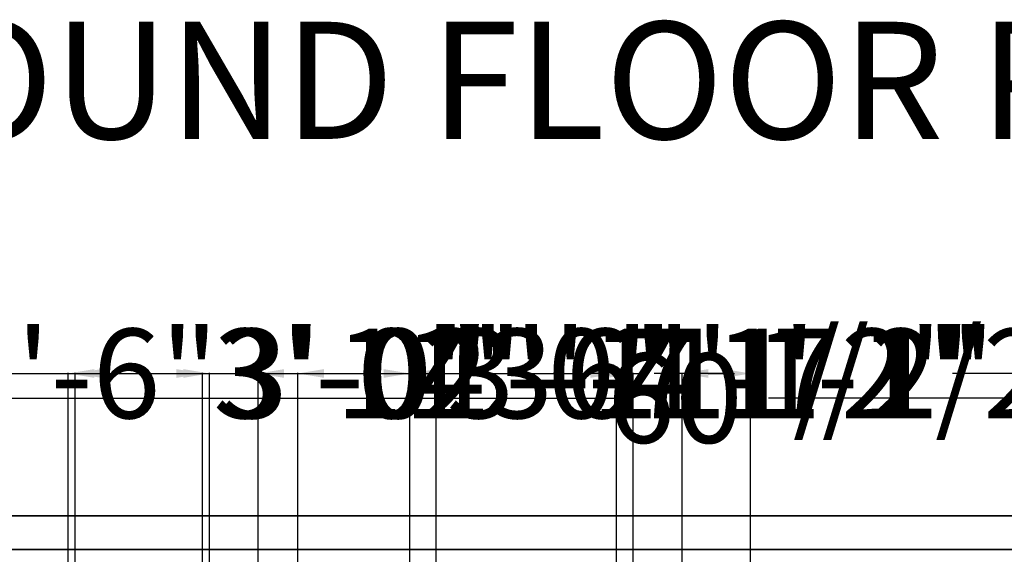
# Model space of a CAD drawing. Units: inches. Extents: x -166 to 1001, y 0 to 688.
# Tile 7 of 11: x 97 to 361, y 544 to 688. Entities that reach past the tile are written whole.
import ezdxf

# ---------------------------------------------------------------- set-up
doc = ezdxf.new("R2010")
doc.units = ezdxf.units.IN
doc.header["$MEASUREMENT"] = 0
for name, color, linetype, lineweight in [('A-ANNO-DIMS', 1, 'Continuous', 18), ('A-ANNO-TEXT', 2, 'Continuous', 25), ('C-SITE-WALL', 250, 'Continuous', 35)]:
    doc.layers.add(name, color=color, linetype=linetype, lineweight=lineweight)
doc.styles.get("Standard").update_dxf_attribs({"font": 'arial.ttf'})
doc.dimstyles.get("Standard").update_dxf_attribs({"dimtxt": 24, "dimasz": 7, "dimexe": 0.18, "dimexo": 0.0625, "dimgap": 0.09, "dimtad": 0, "dimtih": 1, "dimtoh": 1, "dimdec": 0, "dimzin": 0, "dimdsep": 46, "dimlunit": 3, "dimtxsty": 'Standard', "dimcen": 0.09, "dimadec": 0, "dimazin": 0, "dimtfac": 1, "dimtdec": 0, "dimtofl": 0, "dimtmove": 0, "dimatfit": 3, "dimfxl": 1, "dimtolj": 1, "dimtzin": 0, "dimarcsym": 0})

# ---------------------------------------------------------------- blocks, each defined once
blk = doc.blocks.new('*D10')
at = {"layer": 'A-ANNO-DIMS', "color": 0, "lineweight": -2, "transparency": 16777216}
for p, q in [((-82.62, 554.8), (-82.62, 586.48)), ((-75.62, 586.3), (256.61, 586.3)), ((629.88, 586.3), (297.65, 586.3)), ((636.88, 554.8), (636.88, 586.48))]:
    blk.add_line(p, q, dxfattribs=at)
at = {"layer": 'A-ANNO-DIMS', "color": 0, "transparency": 16777216}
for points in [[(-75.62, 587.47), (-75.62, 585.14), (-82.62, 586.3)], [(629.88, 587.47), (629.88, 585.14), (636.88, 586.3)]]:
    blk.add_solid(points, dxfattribs=at)
at = {"layer": 'Defpoints', "color": 0, "transparency": 16777216}
for p in [(636.88, 586.3), (-82.62, 554.74), (636.88, 554.74)]:
    blk.add_point(p, dxfattribs=at)
at = {"layer": 'A-ANNO-DIMS', "color": 0, "transparency": 16777216, "insert": (277.13, 586.3), "char_height": 24, "attachment_point": 5}
blk.add_mtext("\\A1;60'", dxfattribs=at)
blk = doc.blocks.new('*D35')
at = {"layer": 'A-ANNO-DIMS', "color": 0, "lineweight": -2, "transparency": 16777216}
for p, q in [((15.38, 483.8), (15.38, 593.07)), ((22.38, 592.89), (207.38, 592.89)), ((531.88, 592.89), (346.89, 592.89)), ((538.88, 483.8), (538.88, 593.07))]:
    blk.add_line(p, q, dxfattribs=at)
at = {"layer": 'A-ANNO-DIMS', "color": 0, "transparency": 16777216}
for points in [[(22.38, 594.06), (22.38, 591.72), (15.38, 592.89)], [(531.88, 594.06), (531.88, 591.72), (538.88, 592.89)]]:
    blk.add_solid(points, dxfattribs=at)
at = {"layer": 'Defpoints', "color": 0, "transparency": 16777216}
for p in [(538.88, 592.89), (15.38, 483.74), (538.88, 483.74)]:
    blk.add_point(p, dxfattribs=at)
at = {"layer": 'A-ANNO-DIMS', "color": 0, "transparency": 16777216, "insert": (277.13, 592.89), "char_height": 24, "attachment_point": 5}
blk.add_mtext('\\A1;43\'-7 1/2"', dxfattribs=at)
blk = doc.blocks.new('*D43')
at = {"layer": 'A-ANNO-DIMS', "color": 0, "lineweight": -2, "transparency": 16777216}
for p, q in [((160.88, 257.49), (160.88, 593.07)), ((167.88, 592.89), (201.62, 592.89)), ((208.62, 257.49), (208.62, 593.07)), ((208.62, 592.89), (215.62, 592.89))]:
    blk.add_line(p, q, dxfattribs=at)
at = {"layer": 'A-ANNO-DIMS', "color": 0, "transparency": 16777216}
for points in [[(167.88, 594.06), (167.88, 591.72), (160.88, 592.89)], [(201.62, 594.06), (201.62, 591.72), (208.62, 592.89)]]:
    blk.add_solid(points, dxfattribs=at)
at = {"layer": 'Defpoints', "color": 0, "transparency": 16777216}
for p in [(208.62, 592.89), (160.88, 257.42), (208.62, 257.42)]:
    blk.add_point(p, dxfattribs=at)
at = {"layer": 'A-ANNO-DIMS', "color": 0, "transparency": 16777216, "insert": (284.89, 592.89), "char_height": 24, "attachment_point": 5}
blk.add_mtext('\\A1;3\'-11 1/2"', dxfattribs=at)
blk = doc.blocks.new('*D59')
at = {"layer": 'A-ANNO-DIMS', "color": 0, "lineweight": -2, "transparency": 16777216}
for p, q in [((110.03, 342.8), (110.03, 593.07)), ((117.03, 592.89), (139.03, 592.89)), ((146.03, 342.8), (146.03, 593.07)), ((146.03, 592.89), (153.03, 592.89))]:
    blk.add_line(p, q, dxfattribs=at)
at = {"layer": 'A-ANNO-DIMS', "color": 0, "transparency": 16777216}
for points in [[(117.03, 594.06), (117.03, 591.72), (110.03, 592.89)], [(139.03, 594.06), (139.03, 591.72), (146.03, 592.89)]]:
    blk.add_solid(points, dxfattribs=at)
at = {"layer": 'Defpoints', "color": 0, "transparency": 16777216}
for p in [(146.03, 592.89), (110.03, 342.74), (146.03, 342.74)]:
    blk.add_point(p, dxfattribs=at)
at = {"layer": 'A-ANNO-DIMS', "color": 0, "transparency": 16777216, "insert": (185.01, 592.89), "char_height": 24, "attachment_point": 5}
blk.add_mtext('\\A1;3\'-0"', dxfattribs=at)
blk = doc.blocks.new('*D61')
at = {"layer": 'A-ANNO-DIMS', "color": 0, "lineweight": -2, "transparency": 16777216}
for p, q in [((171.55, 342.8), (171.55, 593.07)), ((178.55, 592.89), (194.55, 592.89)), ((201.55, 342.8), (201.55, 593.07)), ((201.55, 592.89), (208.55, 592.89))]:
    blk.add_line(p, q, dxfattribs=at)
at = {"layer": 'A-ANNO-DIMS', "color": 0, "transparency": 16777216}
for points in [[(178.55, 594.06), (178.55, 591.72), (171.55, 592.89)], [(194.55, 594.06), (194.55, 591.72), (201.55, 592.89)]]:
    blk.add_solid(points, dxfattribs=at)
at = {"layer": 'Defpoints', "color": 0, "transparency": 16777216}
for p in [(201.55, 592.89), (171.55, 342.74), (201.55, 342.74)]:
    blk.add_point(p, dxfattribs=at)
at = {"layer": 'A-ANNO-DIMS', "color": 0, "transparency": 16777216, "insert": (240.75, 592.89), "char_height": 24, "attachment_point": 5}
blk.add_mtext('\\A1;2\'-6"', dxfattribs=at)
blk = doc.blocks.new('*D62')
at = {"layer": 'A-ANNO-DIMS', "color": 0, "lineweight": -2, "transparency": 16777216}
for p, q in [((201.55, 342.8), (201.55, 593.07)), ((208.55, 592.89), (249.88, 592.89)), ((256.88, 342.8), (256.88, 593.07)), ((256.88, 592.89), (263.88, 592.89))]:
    blk.add_line(p, q, dxfattribs=at)
at = {"layer": 'A-ANNO-DIMS', "color": 0, "transparency": 16777216}
for points in [[(208.55, 594.06), (208.55, 591.72), (201.55, 592.89)], [(249.88, 594.06), (249.88, 591.72), (256.88, 592.89)]]:
    blk.add_solid(points, dxfattribs=at)
at = {"layer": 'Defpoints', "color": 0, "transparency": 16777216}
for p in [(256.88, 592.89), (201.55, 342.74), (256.88, 342.74)]:
    blk.add_point(p, dxfattribs=at)
at = {"layer": 'A-ANNO-DIMS', "color": 0, "transparency": 16777216, "insert": (324.32, 592.89), "char_height": 24, "attachment_point": 5}
blk.add_mtext('\\A1;4\'-7 1/2"', dxfattribs=at)
blk = doc.blocks.new('*D64')
at = {"layer": 'A-ANNO-DIMS', "color": 0, "lineweight": -2, "transparency": 16777216}
for p, q in [((254.38, 592.89), (247.38, 592.89)), ((261.38, 342.8), (261.38, 593.07)), ((274.49, 342.8), (274.49, 593.07)), ((281.49, 592.89), (288.49, 592.89))]:
    blk.add_line(p, q, dxfattribs=at)
at = {"layer": 'A-ANNO-DIMS', "color": 0, "transparency": 16777216}
for points in [[(254.38, 594.06), (254.38, 591.72), (261.38, 592.89)], [(281.49, 594.06), (281.49, 591.72), (274.49, 592.89)]]:
    blk.add_solid(points, dxfattribs=at)
at = {"layer": 'Defpoints', "color": 0, "transparency": 16777216}
for p in [(274.49, 592.89), (261.38, 342.74), (274.49, 342.74)]:
    blk.add_point(p, dxfattribs=at)
at = {"layer": 'A-ANNO-DIMS', "color": 0, "transparency": 16777216, "insert": (319.35, 592.89), "char_height": 24, "attachment_point": 5}
blk.add_mtext('\\A1;1\'-1"', dxfattribs=at)
blk = doc.blocks.new('*D67')
at = {"layer": 'A-ANNO-DIMS', "color": 0, "lineweight": -2, "transparency": 16777216}
for p, q in [((44.93, 278.3), (44.93, 593.07)), ((51.93, 592.89), (67.93, 592.89)), ((74.93, 278.3), (74.93, 593.07)), ((74.93, 592.89), (81.93, 592.89))]:
    blk.add_line(p, q, dxfattribs=at)
at = {"layer": 'A-ANNO-DIMS', "color": 0, "transparency": 16777216}
for points in [[(51.93, 594.06), (51.93, 591.72), (44.93, 592.89)], [(67.93, 594.06), (67.93, 591.72), (74.93, 592.89)]]:
    blk.add_solid(points, dxfattribs=at)
at = {"layer": 'Defpoints', "color": 0, "transparency": 16777216}
for p in [(74.93, 592.89), (44.93, 278.24), (74.93, 278.24)]:
    blk.add_point(p, dxfattribs=at)
at = {"layer": 'A-ANNO-DIMS', "color": 0, "transparency": 16777216, "insert": (114.12, 592.89), "char_height": 24, "attachment_point": 5}
blk.add_mtext('\\A1;2\'-6"', dxfattribs=at)
blk = doc.blocks.new('*D69')
at = {"layer": 'A-ANNO-DIMS', "color": 0, "lineweight": -2, "transparency": 16777216}
for p, q in [((111.92, 278.3), (111.92, 593.07)), ((118.92, 592.89), (140.87, 592.89)), ((147.87, 278.3), (147.87, 593.07)), ((147.87, 592.89), (154.87, 592.89))]:
    blk.add_line(p, q, dxfattribs=at)
at = {"layer": 'A-ANNO-DIMS', "color": 0, "transparency": 16777216}
for points in [[(118.92, 594.06), (118.92, 591.72), (111.92, 592.89)], [(140.87, 594.06), (140.87, 591.72), (147.87, 592.89)]]:
    blk.add_solid(points, dxfattribs=at)
at = {"layer": 'Defpoints', "color": 0, "transparency": 16777216}
for p in [(147.87, 592.89), (111.92, 278.24), (147.87, 278.24)]:
    blk.add_point(p, dxfattribs=at)
at = {"layer": 'A-ANNO-DIMS', "color": 0, "transparency": 16777216, "insert": (186.85, 592.89), "char_height": 24, "attachment_point": 5}
blk.add_mtext('\\A1;3\'-0"', dxfattribs=at)
blk = doc.blocks.new('*D78')
at = {"layer": 'A-ANNO-DIMS', "color": 0, "lineweight": -2, "transparency": 16777216}
for p, q in [((160.88, 153.8), (160.88, 593.07)), ((167.88, 592.89), (186.64, 592.89)), ((285.77, 592.89), (267.01, 592.89)), ((292.77, 153.8), (292.77, 593.07))]:
    blk.add_line(p, q, dxfattribs=at)
at = {"layer": 'A-ANNO-DIMS', "color": 0, "transparency": 16777216}
for points in [[(167.88, 594.06), (167.88, 591.72), (160.88, 592.89)], [(285.77, 594.06), (285.77, 591.72), (292.77, 592.89)]]:
    blk.add_solid(points, dxfattribs=at)
at = {"layer": 'Defpoints', "color": 0, "transparency": 16777216}
for p in [(292.77, 592.89), (160.88, 153.74), (292.77, 153.74)]:
    blk.add_point(p, dxfattribs=at)
at = {"layer": 'A-ANNO-DIMS', "color": 0, "transparency": 16777216, "insert": (226.83, 592.89), "char_height": 24, "attachment_point": 5}
blk.add_mtext('\\A1;11\'-0"', dxfattribs=at)

msp = doc.modelspace()

# ---------------------------------------------------------------- linework, layer by layer
at = {"layer": 'C-SITE-WALL'}
for p, q in [((-82.62, 554.74), (636.88, 554.74)), ((-73.62, 545.74), (627.88, 545.74))]:
    msp.add_line(p, q, dxfattribs=at)

# ---------------------------------------------------------------- texts
at = {"layer": 'A-ANNO-TEXT'}
msp.add_text('GROUND FLOOR PLAN', height=31.3778, dxfattribs=at).set_placement((17.68, 655.72))

# ---------------------------------------------------------------- dimensions: what is measured, and where the dimension line sits
at = {"layer": 'A-ANNO-DIMS'}
for base, p1, p2, override, picture, middle in [((538.88, 592.89), (15.38, 483.74), (538.88, 483.74), {"dimdec": 1, "dimlfac": 1, "dimrnd": 0, "dimzin": 1, "dimdsep": 46, "dimlunit": 4, "dimfrac": 2}, '*D35', (277.13, 592.89)), ((208.62, 592.89), (160.88, 257.42), (208.62, 257.42), {"dimdec": 1, "dimlfac": 1, "dimrnd": 0, "dimzin": 1, "dimdsep": 46, "dimlunit": 4, "dimfrac": 2}, '*D43', (284.89, 592.89)), ((256.88, 592.89), (201.55, 342.74), (256.88, 342.74), {"dimdec": 1, "dimlfac": 1, "dimrnd": 0, "dimzin": 1, "dimdsep": 46, "dimlunit": 4, "dimfrac": 2}, '*D62', (324.32, 592.89)), ((74.93, 592.89), (44.93, 278.24), (74.93, 278.24), {"dimdec": 1, "dimlfac": 1, "dimrnd": 0, "dimzin": 1, "dimdsep": 46, "dimlunit": 4, "dimfrac": 2}, '*D67', (114.12, 592.89)), ((146.03, 592.89), (110.03, 342.74), (146.03, 342.74), {"dimdec": 1, "dimlfac": 1, "dimrnd": 0, "dimzin": 1, "dimdsep": 46, "dimlunit": 4, "dimfrac": 2}, '*D59', (185.01, 592.89)), ((147.8711, 592.8909), (111.9243, 278.2409), (147.8711, 278.2409), {"dimdec": 1, "dimlfac": 1, "dimrnd": 0, "dimzin": 1, "dimdsep": 46, "dimlunit": 4, "dimfrac": 2}, '*D69', (186.852, 592.8909)), ((292.77, 592.89), (160.88, 153.74), (292.77, 153.74), {"dimdec": 1, "dimlfac": 1, "dimrnd": 0, "dimzin": 1, "dimdsep": 46, "dimlunit": 4, "dimfrac": 2}, '*D78', (226.83, 592.89)), ((201.55, 592.89), (171.55, 342.74), (201.55, 342.74), {"dimdec": 1, "dimlfac": 1, "dimrnd": 0, "dimzin": 1, "dimdsep": 46, "dimlunit": 4, "dimfrac": 2}, '*D61', (240.75, 592.89)), ((274.49, 592.89), (261.38, 342.74), (274.49, 342.74), {"dimdec": 1, "dimlfac": 1, "dimrnd": 0, "dimzin": 1, "dimdsep": 46, "dimlunit": 4, "dimfrac": 2}, '*D64', (319.35, 592.89)), ((636.88246038, 586.30455527), (-82.61753962, 554.740867), (636.88246038, 554.740867), {"dimclrd": 0, "dimclre": 0, "dimclrt": 0}, '*D10', (277.13246038, 586.30455527))]:
    dim = msp.add_linear_dim(base=base, p1=p1, p2=p2, dimstyle='Standard', override=override, dxfattribs=at)
    dim.commit()
    dim.dimension.update_dxf_attribs({"geometry": picture, "text_midpoint": middle})

doc.saveas('drawing.dxf')
